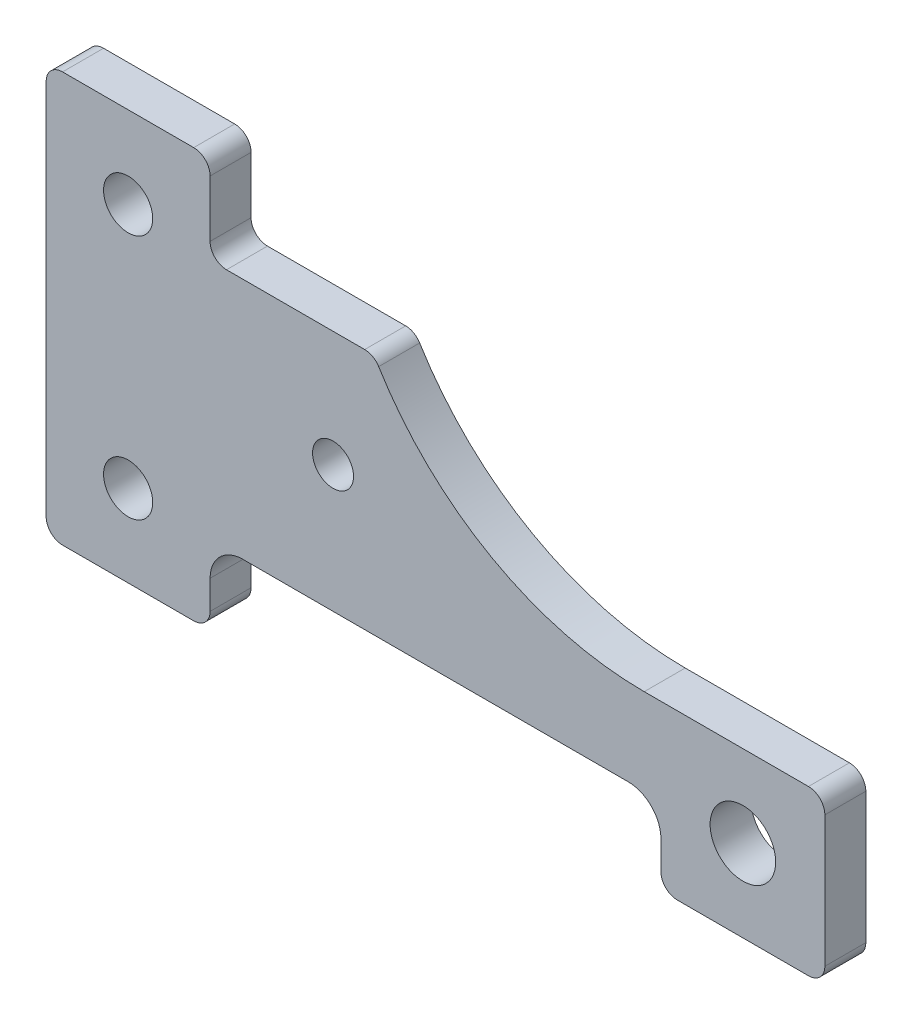
from build123d import *

# Parameters (mm, degrees)
BRACKET_PROFILE_SKETCH_R   = 30
BRACKET_PROFILE_SKETCH_R_2 = 25
BRACKET_PROFILE_SKETCH_R_3 = 40
BRACKET_PLATE_50MM_DEPTH   = 25


with BuildPart() as part:
    # Bracket Profile Sketch → Bracket Plate 50mm (new, symmetric)
    with BuildSketch(Plane.XY):
        with BuildLine():
            Line((-393.337365548, 211.308411215), (-393.337365548, -248.691588785))
            ThreePointArc((-393.337365548, -248.691588785), (-387.479501171, -262.833724409), (-373.337365548, -268.691588785))
            Line((-373.337365548, -268.691588785), (-213.337365548, -268.691588785))
            ThreePointArc((-213.337365548, -268.691588785), (-199.195229924, -262.833724409), (-193.337365548, -248.691588785))
            Line((-193.337365548, -248.691588785), (-193.337365548, -213.676012461))
            ThreePointArc((-193.337365548, -213.676012461), (-181.621636795, -185.391741214), (-153.337365548, -173.676012461))
            Line((-153.337365548, -173.676012461), (316.662634452, -173.676012461))
            ThreePointArc((316.662634452, -173.676012461), (344.9469057, -185.391741214), (356.662634452, -213.676012461))
            Line((356.662634452, -213.676012461), (356.662634452, -248.691588785))
            ThreePointArc((356.662634452, -248.691588785), (362.520498829, -262.833724409), (376.662634452, -268.691588785))
            Line((376.662634452, -268.691588785), (536.662634452, -268.691588785))
            ThreePointArc((536.662634452, -268.691588785), (550.804770076, -262.833724409), (556.662634452, -248.691588785))
            Line((556.662634452, -248.691588785), (556.662634452, -88.691588785))
            ThreePointArc((556.662634452, -88.691588785), (550.804770076, -74.549453161), (536.662634452, -68.691588785))
            Line((536.662634452, -68.691588785), (336.307967431, -68.691588785))
            ThreePointArc((336.307967431, -68.691588785), (150.648831804, -20.2495556), (12.324990963, 112.725856698))
            ThreePointArc((12.324990963, 112.725856698), (5.044788813, 119.724562608), (-4.726744641, 122.274143302))
            Line((-4.726744641, 122.274143302), (-173.337365548, 122.274143302))
            ThreePointArc((-173.337365548, 122.274143302), (-187.479501171, 128.132007678), (-193.337365548, 142.274143302))
            Line((-193.337365548, 142.274143302), (-193.337365548, 211.308411215))
            ThreePointArc((-193.337365548, 211.308411215), (-199.195229924, 225.450546839), (-213.337365548, 231.308411215))
            Line((-213.337365548, 231.308411215), (-373.337365548, 231.308411215))
            ThreePointArc((-373.337365548, 231.308411215), (-387.479501171, 225.450546839), (-393.337365548, 211.308411215))
        make_face()
        with Locations((-293.337365548, 131.308411215)):
            Circle(BRACKET_PROFILE_SKETCH_R, mode=Mode.SUBTRACT)
        with Locations((-293.337365548, -168.691588785)):
            Circle(BRACKET_PROFILE_SKETCH_R, mode=Mode.SUBTRACT)
        with Locations((-43.337365548, -18.691588785)):
            Circle(BRACKET_PROFILE_SKETCH_R_2, mode=Mode.SUBTRACT)
        with Locations((456.662634452, -168.691588785)):
            Circle(BRACKET_PROFILE_SKETCH_R_3, mode=Mode.SUBTRACT)
    extrude(amount=BRACKET_PLATE_50MM_DEPTH, both=True)


solid = part.part
